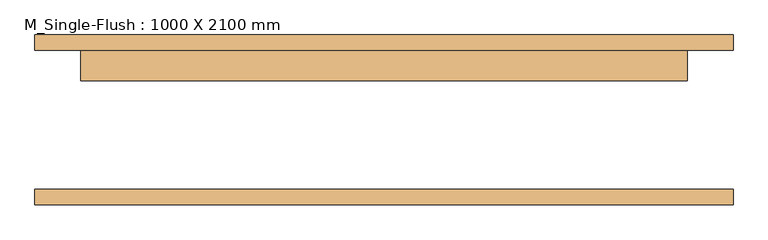
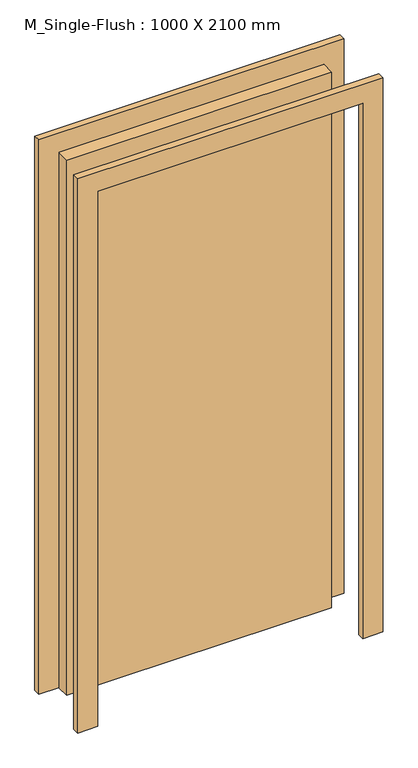
"""IFC4 building model written with IfcOpenShell, lengths in millimetres: door geometry, M_Single-Flush : 1000 X 2100 mm."""

from ifc_helpers import new_model, si_unit, frame, origin, origin_with_axes, place, context, project, spatial, polyline, outline, extrude, source, transform, mapped, element, save


def m_single_flush_1000_x_2100_mm_10f5ba11(model_context):
    return source(origin(), model_context, "Body", "SweptSolid", [
        extrude(outline(polyline([(2210.0, -576.0), (0.0, -576.0), (0.0, -500.0), (2134.0, -500.0), (2134.0, 500.0), (0.0, 500.0), (0.0, 576.0), (2210.0, 576.0), (2210.0, -576.0)])), frame((0.0, 115.0, 0.0), z_axis=(0.0, 1.0, 0.0), x_axis=(0.0, 0.0, 1.0)), (0.0, 0.0, 1.0), 25.0),
        extrude(outline(polyline([(2210.0, 576.0), (2210.0, -576.0), (0.0, -576.0), (0.0, -500.0), (2134.0, -500.0), (2134.0, 500.0), (0.0, 500.0), (0.0, 576.0), (2210.0, 576.0)])), frame((0.0, -140.0, 0.0), z_axis=(0.0, 1.0, 0.0), x_axis=(0.0, 0.0, 1.0)), (0.0, 0.0, 1.0), 25.0),
        extrude(outline(polyline([(500.0, 64.0), (-500.0, 64.0), (-500.0, 115.0), (500.0, 115.0), (500.0, 64.0)])), origin_with_axes(), (0.0, 0.0, 1.0), 2134.0),
    ])


if __name__ == "__main__":
    model = new_model("IFC4")
    model_context = context("Model", 3, world=origin())
    ifc_project = project(units=[si_unit("LENGTHUNIT", "METRE", prefix="MILLI")], contexts=[model_context])
    site = spatial("IfcSite", under=ifc_project)
    building = spatial("IfcBuilding", under=site)
    placement = place(None, origin())
    m_single_flush_1000_x_2100_mm_shape = m_single_flush_1000_x_2100_mm_10f5ba11(model_context)
    element("IfcDoor", 1, ObjectType="M_Single-Flush : 1000 X 2100 mm", at=placement, inside=building, context=model_context, shape_type="MappedRepresentation", body=[
        mapped(m_single_flush_1000_x_2100_mm_shape, transform((0.0, 0.0, 0.0), x_axis=(1.0, 0.0, 0.0), y_axis=(0.0, 1.0, 0.0), z_axis=(0.0, 0.0, 1.0))),
    ])
    save(model, "model.ifc")

# Revit data of these elements
# Type "M_Single-Flush : 1000 X 2100 mm"
#   Type Mark = "40"
#   Construction Type Id = "MDOOR"
#   Analytic Construction = "Metal"
#   Thickness = 0.051 m
#   Thermal Resistance (R) = 0.270117 (m²·K)/W
#   Heat Transfer Coefficient (U) = 3.7021 W/(m²·K)
#   Height = 2.134 m
#   Trim Projection Ext = 0.025 m
#   Trim Projection Int = 0.025 m
#   Trim Width = 0.076 m
#   Width = 1 m
#   Define Thermal Properties by = 1
#   Door Material = Door - Panel
#   Frame Material = Door - Frame
#   Visual Light Transmittance = 0
#   Solar Heat Gain Coefficient = 0
#   Function = (empty or 0)
#   Wall Closure = (empty or 0)
# Element 1 (IfcDoor, "M_Single-Flush : 1000 X 2100 mm")
#   Materials on its faces: "Door - Frame", "Door - Panel"
# Materials
#   "Door - Panel": class "Wood", colour RGB 210 159 95, transparency 0, Cost = 0
#   "Door - Frame": colour RGB 118 70 51, transparency 0, Cost = 0
